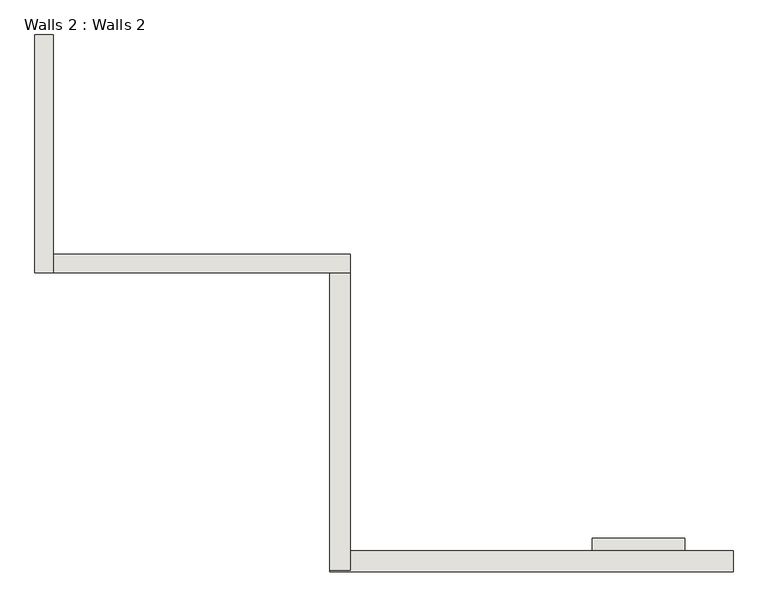
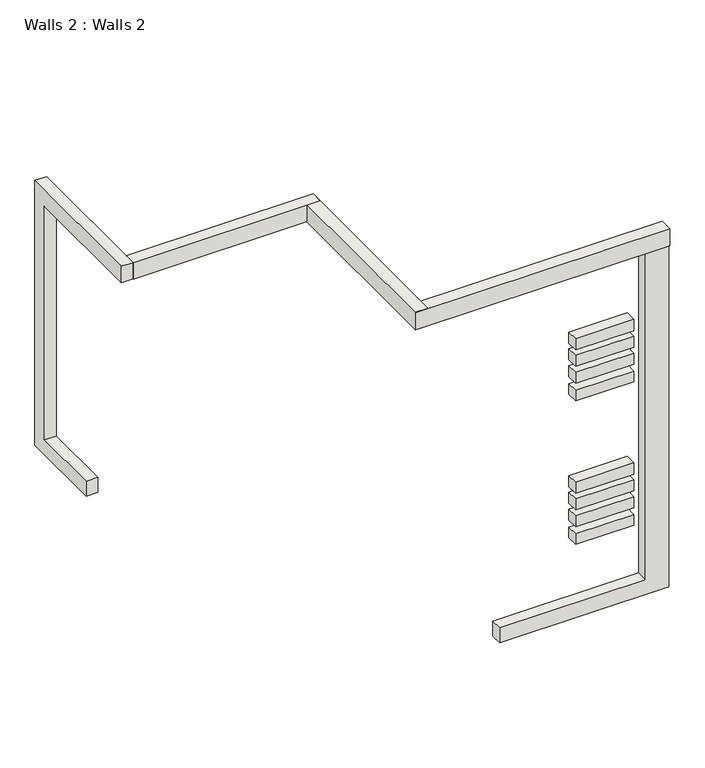
"""IFC4 building model written with IfcOpenShell, lengths in millimetres: wall geometry, Walls 2 : Walls 2."""

from ifc_helpers import new_model, si_unit, frame, origin, place, context, project, spatial, polyline, outline, extrude, source, transform, mapped, element, save


def walls_2_walls_2_327077e9(model_context):
    return source(origin(), model_context, "Body", "SweptSolid", [
        extrude(outline(polyline([(-2171.7239145, -754.1387835), (-3695.7239145, -754.1387835), (-3695.7239145, -449.3387835), (-2171.7239145, -449.3387835), (-2171.7239145, -754.1387835)])), frame((0.0, 0.0, 8598.0489127), z_axis=(0.0, 0.0, 1.0), x_axis=(1.0, 0.0, 0.0)), (0.0, 0.0, 1.0), 304.8),
        extrude(outline(polyline([(-2171.7239145, -754.1387835), (-3695.7239145, -754.1387835), (-3695.7239145, -449.3387835), (-2171.7239145, -449.3387835), (-2171.7239145, -754.1387835)])), frame((0.0, 0.0, 8140.8489127), z_axis=(0.0, 0.0, 1.0), x_axis=(1.0, 0.0, 0.0)), (0.0, 0.0, 1.0), 304.8),
        extrude(outline(polyline([(-2171.7239145, -754.1387835), (-3695.7239145, -754.1387835), (-3695.7239145, -449.3387835), (-2171.7239145, -449.3387835), (-2171.7239145, -754.1387835)])), frame((0.0, 0.0, 7670.8), z_axis=(0.0, 0.0, 1.0), x_axis=(1.0, 0.0, 0.0)), (0.0, 0.0, 1.0), 304.8),
        extrude(outline(polyline([(-2171.7239145, -754.1387835), (-3695.7239145, -754.1387835), (-3695.7239145, -449.3387835), (-2171.7239145, -449.3387835), (-2171.7239145, -754.1387835)])), frame((0.0, 0.0, 7188.913627), z_axis=(0.0, 0.0, 1.0), x_axis=(1.0, 0.0, 0.0)), (0.0, 0.0, 1.0), 289.9423012),
        extrude(outline(polyline([(-2171.7239145, -754.1387835), (-3695.7239145, -754.1387835), (-3695.7239145, -449.3387835), (-2171.7239145, -449.3387835), (-2171.7239145, -754.1387835)])), frame((0.0, 0.0, 4635.6489127), z_axis=(0.0, 0.0, 1.0), x_axis=(1.0, 0.0, 0.0)), (0.0, 0.0, 1.0), 304.8),
        extrude(outline(polyline([(-2171.7239145, -754.1387835), (-3695.7239145, -754.1387835), (-3695.7239145, -449.3387835), (-2171.7239145, -449.3387835), (-2171.7239145, -754.1387835)])), frame((0.0, 0.0, 4178.4489127), z_axis=(0.0, 0.0, 1.0), x_axis=(1.0, 0.0, 0.0)), (0.0, 0.0, 1.0), 304.8),
        extrude(outline(polyline([(-2171.7239145, -754.1387835), (-3695.7239145, -754.1387835), (-3695.7239145, -449.3387835), (-2171.7239145, -449.3387835), (-2171.7239145, -754.1387835)])), frame((0.0, 0.0, 3708.4), z_axis=(0.0, 0.0, 1.0), x_axis=(1.0, 0.0, 0.0)), (0.0, 0.0, 1.0), 304.8),
        extrude(outline(polyline([(-2171.7239145, -754.1387835), (-3695.7239145, -754.1387835), (-3695.7239145, -449.3387835), (-2171.7239145, -449.3387835), (-2171.7239145, -754.1387835)])), frame((0.0, 0.0, 3226.513627), z_axis=(0.0, 0.0, 1.0), x_axis=(1.0, 0.0, 0.0)), (0.0, 0.0, 1.0), 289.9423012),
        extrude(outline(polyline([(1371.6, -1380.4681702), (10972.8, -1380.4681702), (10972.8, -1990.0681702), (1778.0, -1990.0681702), (1778.0, -5800.0681702), (1371.6, -5800.0681702), (1371.6, -1380.4681702)])), frame((0.0, -957.3387835, 0.0), z_axis=(0.0, 1.0, 0.0), x_axis=(0.0, 0.0, 1.0)), (0.0, 0.0, 1.0), 304.8),
        extrude(outline(polyline([(7831.0612165, 11277.6), (7831.0612165, 3962.4), (5517.1742715, 3962.4), (5517.1742715, 4375.6027373), (7399.8573992, 4375.6027373), (7399.8573992, 10825.2489869), (3919.4612165, 10825.2489869), (3919.4612165, 11277.6), (7831.0612165, 11277.6)])), frame((-12861.2681702, 0.0, 0.0), z_axis=(1.0, 0.0, 0.0), x_axis=(0.0, 1.0, 0.0)), (0.0, 0.0, 1.0), 304.8),
        extrude(outline(polyline([(-7679.6681702, 3919.4612165), (-12556.4681702, 3919.4612165), (-12556.4681702, 4224.2612165), (-7679.6681702, 4224.2612165), (-7679.6681702, 3919.4612165)])), frame((0.0, 0.0, 10816.7212722), z_axis=(0.0, 0.0, 1.0), x_axis=(1.0, 0.0, 0.0)), (0.0, 0.0, 1.0), 460.8787278),
        extrude(outline(polyline([(-8013.9109677, -972.404839), (-8013.9109677, 4224.2612165), (-7679.6681702, 4224.2612165), (-7679.6681702, -972.404839), (-8013.9109677, -972.404839)])), frame((0.0, 0.0, 10801.9794049), z_axis=(0.0, 0.0, 1.0), x_axis=(1.0, 0.0, 0.0)), (0.0, 0.0, 1.0), 475.6205951),
        extrude(outline(polyline([(-1380.4681702, -995.9471159), (-8010.6534973, -995.9471159), (-8010.6534973, -652.5387835), (-1380.4681702, -652.5387835), (-1380.4681702, -995.9471159)])), frame((0.0, 0.0, 10808.5899371), z_axis=(0.0, 0.0, 1.0), x_axis=(1.0, 0.0, 0.0)), (0.0, 0.0, 1.0), 469.0100629),
    ])


if __name__ == "__main__":
    model = new_model("IFC4")
    model_context = context("Model", 3, world=origin())
    ifc_project = project(units=[si_unit("LENGTHUNIT", "METRE", prefix="MILLI")], contexts=[model_context])
    site = spatial("IfcSite", under=ifc_project)
    building = spatial("IfcBuilding", under=site)
    placement = place(None, origin())
    walls_2_walls_2_shape = walls_2_walls_2_327077e9(model_context)
    element("IfcWall", 1, ObjectType="Walls 2 : Walls 2", at=placement, inside=building, context=model_context, shape_type="MappedRepresentation", body=[
        mapped(walls_2_walls_2_shape, transform((0.0, 0.0, 0.0), x_axis=(1.0, 0.0, 0.0), y_axis=(0.0, 1.0, 0.0), z_axis=(0.0, 0.0, 1.0))),
    ])
    save(model, "model.ifc")

# Revit data of these elements
# Element 1 (IfcWall, "Walls 2 : Walls 2")
#   Materials on its faces: "Default Wall"
# Materials
#   "Default Wall": colour RGB 128 128 128, transparency 0
